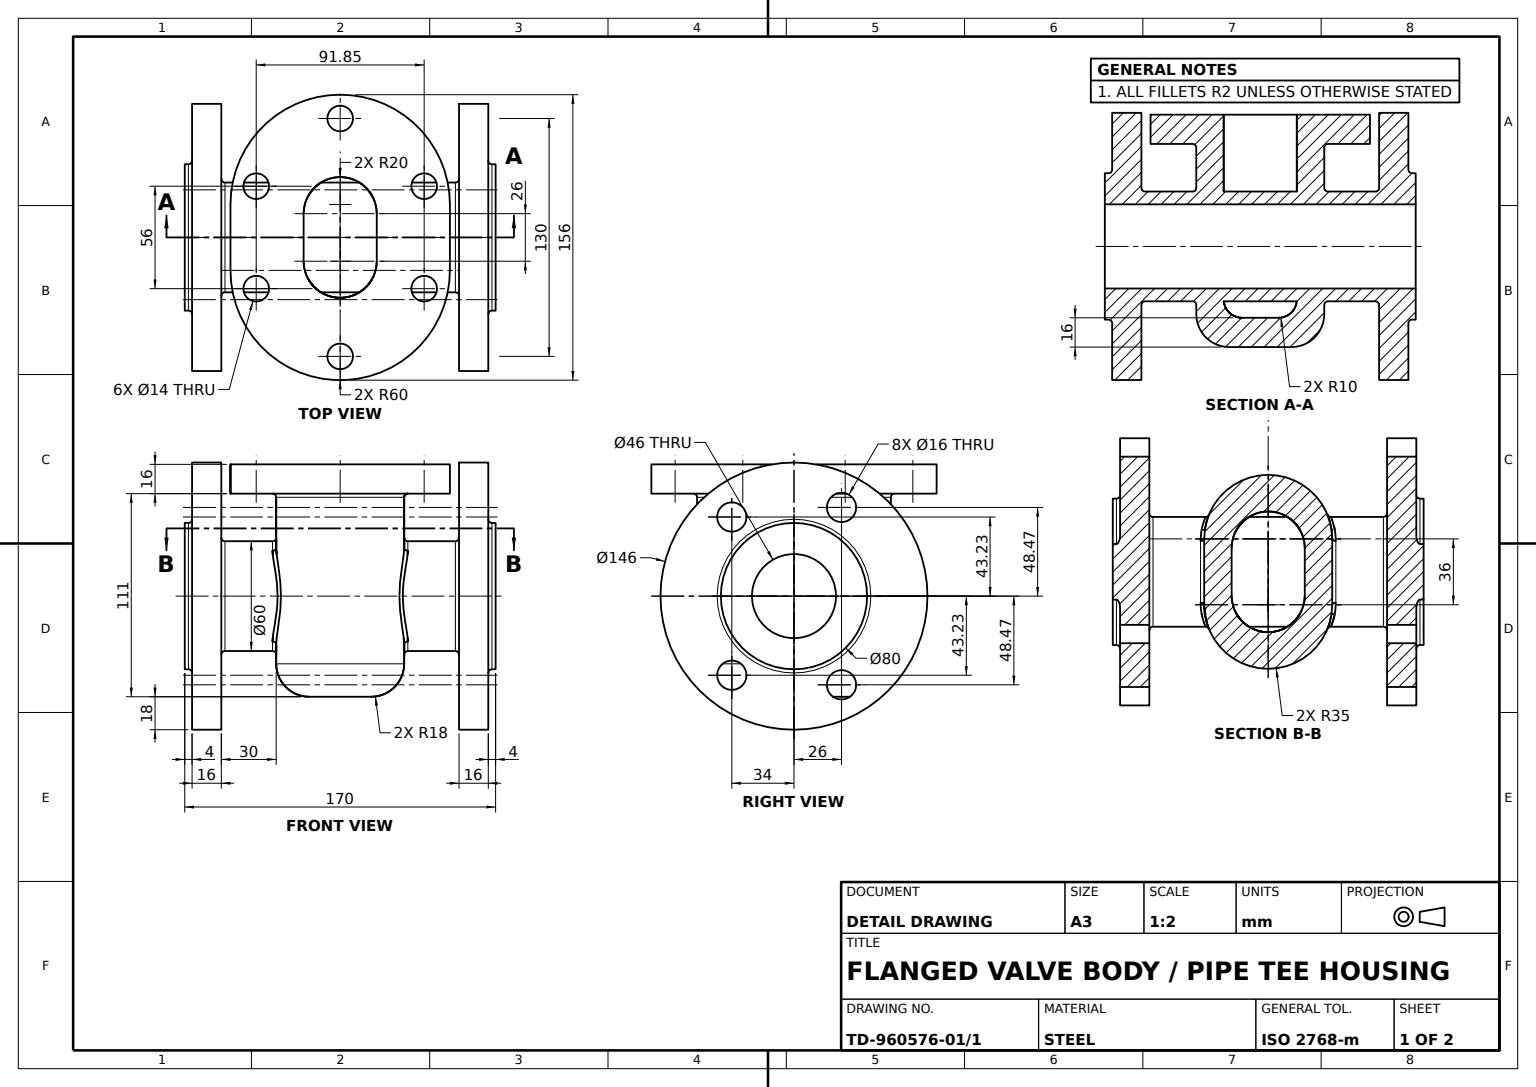
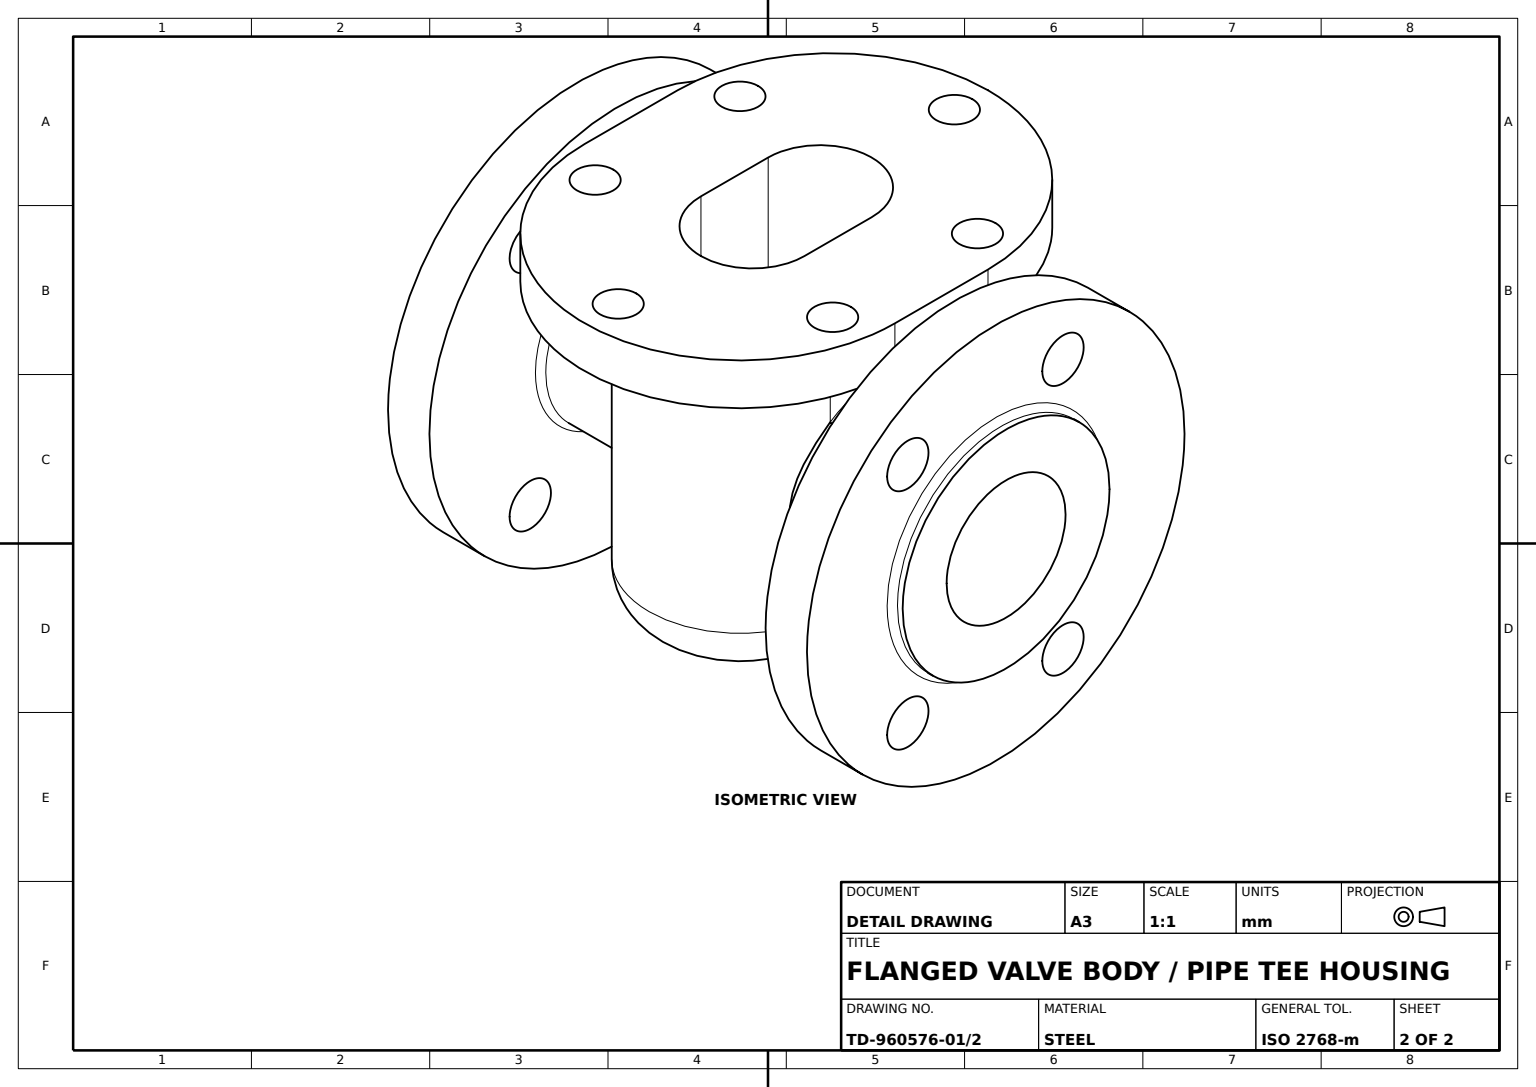
from build123d import *

# Parameters (mm, degrees)
BONNET_FLANGE_SKETCH_R     = 7
BONNET_FLANGE_DEPTH        = 16
NECK_DEPTH                 = 111
NECK_SLOT_BORE_DEPTH       = 111
NECK_EDGE_FILLET_R18_R     = 18
SLOT_BORE_FILLET_R10_R     = 10
END_FLANGE_SKETCH_R        = 73
END_FLANGE_146_DEPTH       = 16
BARREL_SKETCH_R            = 30
BARREL_60_DEPTH            = 148
RAISED_FACE_A_SKETCH_R     = 40
RAISED_FACE_A_80_DEPTH     = 4
RAISED_START               = 4
RAISED_FACE_B_SKETCH_R     = 40
RAISED_FACE_B_80_DEPTH     = 4
THROUGH_BORE_SKETCH_R      = 23
THROUGH_BORE_46_DEPTH      = 174
RAISED_FACE_FILLETS_R2_R   = 2
BARREL_FLANGE_FILLETS_R2_R = 2
FLANGE_BOLT_HOLES_SKETCH_R = 8
FLANGE_BOLT_HOLES_DEPTH    = 16
NECK_BONNET_FILLET_R2_R    = 2
NECK_BARREL_FILLET_R2_R    = 2


with BuildPart() as part:
    # Bonnet Flange Sketch → Bonnet Flange (new body)
    with BuildSketch(Plane(origin=(0, 0, 0), x_dir=(1, 0, 0), z_dir=(0, 1, 0))):
        with BuildLine():
            Line((-60, -18), (-60, 18))
            ThreePointArc((-60, 18), (0, 78), (60, 18))
            Line((60, 18), (60, -18))
            ThreePointArc((60, -18), (0, -78), (-60, -18))
        make_face()
        with Locations(Location((0, 65, 0), (0, 0, 270))):
            Circle(BONNET_FLANGE_SKETCH_R, mode=Mode.SUBTRACT)
        with Locations(Location((0, -65, 0), (0, 0, 270))):
            Circle(BONNET_FLANGE_SKETCH_R, mode=Mode.SUBTRACT)
        with Locations(Location((45.923850013, 28, 0), (0, 0, 270))):
            Circle(BONNET_FLANGE_SKETCH_R, mode=Mode.SUBTRACT)
        with Locations(Location((45.923850013, -28, 0), (0, 0, 270))):
            Circle(BONNET_FLANGE_SKETCH_R, mode=Mode.SUBTRACT)
        with Locations(Location((-45.923850013, 28, 0), (0, 0, 90))):
            Circle(BONNET_FLANGE_SKETCH_R, mode=Mode.SUBTRACT)
        with Locations(Location((-45.923850013, -28, 0), (0, 0, 90))):
            Circle(BONNET_FLANGE_SKETCH_R, mode=Mode.SUBTRACT)
    extrude(amount=BONNET_FLANGE_DEPTH)

    # Neck Sketch → Neck (add)
    with BuildSketch(Plane.XZ):
        with BuildLine():
            Line((-35, -18), (-35, 18))
            ThreePointArc((-35, 18), (0, 53), (35, 18))
            Line((35, 18), (35, -18))
            ThreePointArc((35, -18), (0, -53), (-35, -18))
        make_face()
    extrude(amount=NECK_DEPTH)

    # Neck Slot Bore Sketch → Neck Slot Bore (cut)
    with BuildSketch(Plane(origin=(0, 16, 0), x_dir=(1, 0, 0), z_dir=(0, 1, 0))):
        with BuildLine():
            Line((-20, -13), (-20, 13))
            ThreePointArc((-20, 13), (0, 33), (20, 13))
            Line((20, 13), (20, -13))
            ThreePointArc((20, -13), (0, -33), (-20, -13))
        make_face()
    extrude(amount=-NECK_SLOT_BORE_DEPTH, mode=Mode.SUBTRACT)

    # Neck Edge Fillet R18
    neck_edge_fillet_r18_edges = [part.edges().sort_by_distance(p)[0] for p in [
        (-35, -111, 0),
        (0, -111, -53),
        (35, -111, 0),
        (0, -111, 53),
    ]]
    fillet(neck_edge_fillet_r18_edges, radius=NECK_EDGE_FILLET_R18_R)

    # Slot Bore Fillet R10
    slot_bore_fillet_r10_edges = [part.edges().sort_by_distance(p)[0] for p in [
        (0, -95, 33),
        (-20, -95, 0),
        (0, -95, -33),
        (20, -95, 0),
    ]]
    fillet(slot_bore_fillet_r10_edges, radius=SLOT_BORE_FILLET_R10_R)



with BuildPart() as body_2:
    # End Flange Sketch → End Flange Ø146 (new body)
    with BuildSketch(Plane(origin=(81, 0, 0), x_dir=(0, 0, -1), z_dir=(1, 0, 0))):
        with Locations((0, -56)):
            Circle(END_FLANGE_SKETCH_R)
    extrude(amount=-END_FLANGE_146_DEPTH)


with BuildPart() as body_3:
    # Opposite End Flange Mirror: mirrored copy
    add(body_2.part.mirror(Plane(origin=(0, 0, 0), x_dir=(0, 0, 1), z_dir=(1, 0, 0))))


with BuildPart() as part_1:
    add(part.part)

    add(body_2.part)  # Barrel Ø60 merges body 2

    add(body_3.part)  # Barrel Ø60 merges body 3
    # Barrel Sketch → Barrel Ø60 (add)
    with BuildSketch(Plane(origin=(81, 0, 0), x_dir=(0, 0, -1), z_dir=(1, 0, 0))):
        with Locations(Location((0, -56, 0), (0, 0, 306.869897646))):
            Circle(BARREL_SKETCH_R)
    extrude(amount=-BARREL_60_DEPTH)

    # Raised Face A Sketch → Raised Face A Ø80 (add)
    with BuildSketch(Plane(origin=(81, 0, 0), x_dir=(0, 0, -1), z_dir=(1, 0, 0))):
        with Locations((0, -56)):
            Circle(RAISED_FACE_A_SKETCH_R)
    extrude(amount=RAISED_FACE_A_80_DEPTH)

    # Raised Face B Sketch → Raised Face B Ø80 (add)
    with BuildSketch(Plane.ZY.offset(81).offset(RAISED_START)):
        with Locations(Location((0, -56, 0), (0, 0, 180))):
            Circle(RAISED_FACE_B_SKETCH_R)
    extrude(amount=-RAISED_FACE_B_80_DEPTH)

    # Through Bore Sketch → Through Bore Ø46 (cut)
    with BuildSketch(Plane.ZY.offset(85)):
        with Locations((0, -56)):
            Circle(THROUGH_BORE_SKETCH_R)
    extrude(amount=-THROUGH_BORE_46_DEPTH, mode=Mode.SUBTRACT)

    # Raised Face Fillets R2
    raised_face_fillets_r2_edges = [part_1.edges().sort_by_distance(p)[0] for p in [
        (81, -56, 40),
        (-81, -56, 40),
    ]]
    fillet(raised_face_fillets_r2_edges, radius=RAISED_FACE_FILLETS_R2_R)

    # Barrel Flange Fillets R2
    barrel_flange_fillets_r2_edges = [part_1.edges().sort_by_distance(p)[0] for p in [
        (65, -32, 18),
        (-65, -32, 18),
    ]]
    fillet(barrel_flange_fillets_r2_edges, radius=BARREL_FLANGE_FILLETS_R2_R)

    # Flange Bolt Holes Sketch → Flange Bolt Holes (cut)
    with BuildSketch(Plane(origin=(81, 0, 0), x_dir=(0, 0, -1), z_dir=(1, 0, 0))):
        with Locations((26, -104.466483264)):
            Circle(FLANGE_BOLT_HOLES_SKETCH_R)
        with Locations((-34, -99.231932642)):
            Circle(FLANGE_BOLT_HOLES_SKETCH_R)
        with Locations(Location((-34, -12.768067358, 0), (0, 0, 180))):
            Circle(FLANGE_BOLT_HOLES_SKETCH_R)
        with Locations(Location((26, -7.533516736, 0), (0, 0, 180))):
            Circle(FLANGE_BOLT_HOLES_SKETCH_R)
    flange_bolt_holes = extrude(amount=-FLANGE_BOLT_HOLES_DEPTH, mode=Mode.SUBTRACT)

    # Flange Bolt Holes Mirror: Flange Bolt Holes across plane
    add(flange_bolt_holes.mirror(Plane(origin=(0, 0, 0), x_dir=(0, 0, 1), z_dir=(1, 0, 0))), mode=Mode.SUBTRACT)

    # Neck Bonnet Fillet R2
    neck_bonnet_fillet_r2_edges = [part_1.edges().sort_by_distance(p)[0] for p in [
        (0, 0, -53),
        (35, 0, 0),
        (0, 0, 53),
        (-35, 0, 0),
    ]]
    fillet(neck_bonnet_fillet_r2_edges, radius=NECK_BONNET_FILLET_R2_R)

    # Neck Barrel Fillet R2
    neck_barrel_fillet_r2_edges = [part_1.edges().sort_by_distance(p)[0] for p in [
        (-35, -86, 0),
        (-35, -26, 0),
        (35, -26, 0),
        (32.878564446, -56, -30),
        (35, -86, 0),
        (32.878564446, -56, 30),
        (-32.878564446, -56, -30),
        (-32.878564446, -56, 30),
    ]]
    fillet(neck_barrel_fillet_r2_edges, radius=NECK_BARREL_FILLET_R2_R)


solid = part_1.part
